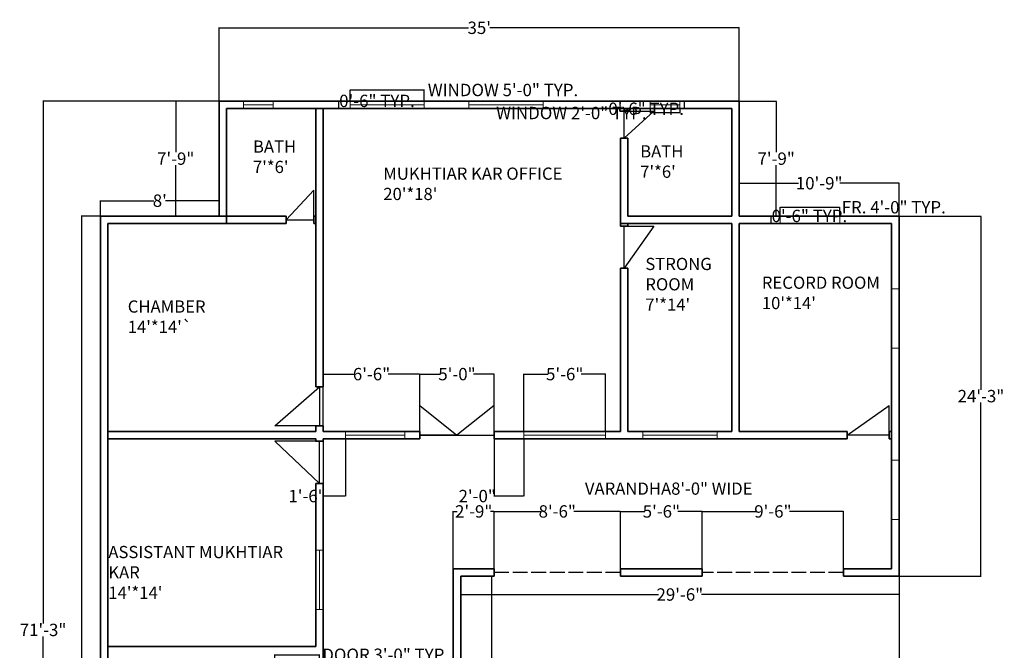
# Model space of a CAD drawing. Units: inches. Extents: x 20 to 815, y -31 to 943.
# Tile 2 of 2: x 20 to 815, y 433 to 943. Entities that reach past the tile are written whole.
import ezdxf

# ---------------------------------------------------------------- set-up
doc = ezdxf.new("R2010")
doc.units = ezdxf.units.IN
doc.header["$MEASUREMENT"] = 0
doc.linetypes.add('ACAD_ISO02W100', pattern=[15, 12, -3])
for name, color, linetype, lineweight in [('A-ANNO-DIMS', 2, 'Continuous', 18), ('A-AREA-IDEN', 7, 'Continuous', 18), ('A-DOOR', 3, 'Continuous', 25), ('A-FLOR-GRIL', 8, 'ACAD_ISO02W100', 25), ('A-GLAZ', 4, 'Continuous', 18), ('A-WALL', 7, 'Continuous', 35)]:
    doc.layers.add(name, color=color, linetype=linetype, lineweight=lineweight)
doc.styles.get("Standard").update_dxf_attribs({"font": 'arial.ttf'})
doc.dimstyles.get("Standard").update_dxf_attribs({"dimtxt": 10, "dimasz": 0.18, "dimexe": 0.18, "dimexo": 0.0625, "dimgap": 0.09, "dimtad": 0, "dimtih": 1, "dimtoh": 1, "dimdec": 0, "dimzin": 0, "dimdsep": 46, "dimlunit": 3, "dimtxsty": 'Standard', "dimcen": 0.09, "dimadec": 0, "dimazin": 0, "dimtfac": 1, "dimtdec": 0, "dimtofl": 0, "dimtmove": 0, "dimatfit": 3, "dimfxl": 1, "dimtolj": 1, "dimtzin": 0, "dimarcsym": 0})

# ---------------------------------------------------------------- blocks, each defined once
blk = doc.blocks.new('*D1')
at = {"layer": 'A-ANNO-DIMS', "color": 0, "lineweight": -2, "transparency": 16777216}
for p, q in [((181.05, 877.05), (181.05, 936.45)), ((181.23, 936.27), (382.48, 936.27)), ((600.87, 936.27), (399.62, 936.27)), ((601.05, 877.05), (601.05, 936.45))]:
    blk.add_line(p, q, dxfattribs=at)
at = {"layer": 'A-ANNO-DIMS', "color": 0, "transparency": 16777216}
for points in [[(181.23, 936.3), (181.23, 936.24), (181.05, 936.27)], [(600.87, 936.3), (600.87, 936.24), (601.05, 936.27)]]:
    blk.add_solid(points, dxfattribs=at)
at = {"layer": 'Defpoints', "color": 0, "transparency": 16777216}
for p in [(601.05, 936.27), (181.05, 876.99), (601.05, 876.99)]:
    blk.add_point(p, dxfattribs=at)
at = {"layer": 'A-ANNO-DIMS', "color": 0, "transparency": 16777216, "insert": (391.05, 936.27), "char_height": 10, "attachment_point": 5}
blk.add_mtext("\\A1;35'", dxfattribs=at)
blk = doc.blocks.new('*D2')
at = {"layer": 'A-ANNO-DIMS', "color": 0, "lineweight": -2, "transparency": 16777216}
for p, q in [((601.11, 876.99), (631.03, 876.99)), ((630.85, 876.81), (630.85, 835.69)), ((630.85, 784.17), (630.85, 825.3)), ((601.11, 783.99), (631.03, 783.99))]:
    blk.add_line(p, q, dxfattribs=at)
at = {"layer": 'A-ANNO-DIMS', "color": 0, "transparency": 16777216}
for points in [[(630.82, 876.81), (630.88, 876.81), (630.85, 876.99)], [(630.82, 784.17), (630.88, 784.17), (630.85, 783.99)]]:
    blk.add_solid(points, dxfattribs=at)
at = {"layer": 'Defpoints', "color": 0, "transparency": 16777216}
for p in [(601.05, 876.99), (601.05, 783.99), (630.85, 783.99)]:
    blk.add_point(p, dxfattribs=at)
at = {"layer": 'A-ANNO-DIMS', "color": 0, "transparency": 16777216, "insert": (630.85, 830.49), "char_height": 10, "attachment_point": 5}
blk.add_mtext('\\A1;7\'-9"', dxfattribs=at)
blk = doc.blocks.new('*D3')
at = {"layer": 'A-ANNO-DIMS', "color": 0, "lineweight": -2, "transparency": 16777216}
for p, q in [((601.05, 784.05), (601.05, 810.82)), ((601.23, 810.64), (648.76, 810.64)), ((729.87, 810.64), (682.35, 810.64)), ((730.05, 784.05), (730.05, 810.82))]:
    blk.add_line(p, q, dxfattribs=at)
at = {"layer": 'A-ANNO-DIMS', "color": 0, "transparency": 16777216}
for points in [[(601.23, 810.67), (601.23, 810.61), (601.05, 810.64)], [(729.87, 810.67), (729.87, 810.61), (730.05, 810.64)]]:
    blk.add_solid(points, dxfattribs=at)
at = {"layer": 'Defpoints', "color": 0, "transparency": 16777216}
for p in [(730.05, 810.64), (601.05, 783.99), (730.05, 783.99)]:
    blk.add_point(p, dxfattribs=at)
at = {"layer": 'A-ANNO-DIMS', "color": 0, "transparency": 16777216, "insert": (665.55, 810.64), "char_height": 10, "attachment_point": 5}
blk.add_mtext('\\A1;10\'-9"', dxfattribs=at)
blk = doc.blocks.new('*D4')
at = {"layer": 'A-ANNO-DIMS', "color": 0, "lineweight": -2, "transparency": 16777216}
for p, q in [((730.11, 783.99), (796.4, 783.99)), ((796.22, 783.81), (796.22, 643.69)), ((796.22, 493.17), (796.22, 633.29)), ((730.11, 492.99), (796.4, 492.99))]:
    blk.add_line(p, q, dxfattribs=at)
at = {"layer": 'A-ANNO-DIMS', "color": 0, "transparency": 16777216}
for points in [[(796.19, 783.81), (796.25, 783.81), (796.22, 783.99)], [(796.19, 493.17), (796.25, 493.17), (796.22, 492.99)]]:
    blk.add_solid(points, dxfattribs=at)
at = {"layer": 'Defpoints', "color": 0, "transparency": 16777216}
for p in [(730.05, 783.99), (796.22, 783.99), (730.05, 492.99)]:
    blk.add_point(p, dxfattribs=at)
at = {"layer": 'A-ANNO-DIMS', "color": 0, "transparency": 16777216, "insert": (796.22, 638.49), "char_height": 10, "attachment_point": 5}
blk.add_mtext('\\A1;24\'-3"', dxfattribs=at)
blk = doc.blocks.new('*D5')
at = {"layer": 'A-ANNO-DIMS', "color": 0, "lineweight": -2, "transparency": 16777216}
for p, q in [((376.05, 492.93), (376.05, 477.94)), ((730.05, 492.93), (730.05, 477.94)), ((376.23, 478.12), (535.7, 478.12)), ((729.87, 478.12), (570.4, 478.12))]:
    blk.add_line(p, q, dxfattribs=at)
at = {"layer": 'A-ANNO-DIMS', "color": 0, "transparency": 16777216}
for points in [[(376.23, 478.15), (376.23, 478.09), (376.05, 478.12)], [(729.87, 478.15), (729.87, 478.09), (730.05, 478.12)]]:
    blk.add_solid(points, dxfattribs=at)
at = {"layer": 'Defpoints', "color": 0, "transparency": 16777216}
for p in [(376.05, 492.99), (730.05, 492.99), (376.05, 478.12)]:
    blk.add_point(p, dxfattribs=at)
at = {"layer": 'A-ANNO-DIMS', "color": 0, "transparency": 16777216, "insert": (553.05, 478.12), "char_height": 10, "attachment_point": 5}
blk.add_mtext('\\A1;29\'-6"', dxfattribs=at)
blk = doc.blocks.new('*D6')
at = {"layer": 'A-ANNO-DIMS', "color": 0, "lineweight": -2, "transparency": 16777216}
for p, q in [((84.99, 783.99), (69.56, 783.99)), ((69.74, 783.81), (69.74, 408.19)), ((69.74, 22.17), (69.74, 397.79)), ((84.99, 21.99), (69.56, 21.99))]:
    blk.add_line(p, q, dxfattribs=at)
at = {"layer": 'A-ANNO-DIMS', "color": 0, "transparency": 16777216}
for points in [[(69.71, 783.81), (69.77, 783.81), (69.74, 783.99)], [(69.71, 22.17), (69.77, 22.17), (69.74, 21.99)]]:
    blk.add_solid(points, dxfattribs=at)
at = {"layer": 'Defpoints', "color": 0, "transparency": 16777216}
for p in [(69.74, 783.99), (85.05, 783.99), (85.05, 21.99)]:
    blk.add_point(p, dxfattribs=at)
at = {"layer": 'A-ANNO-DIMS', "color": 0, "transparency": 16777216, "insert": (69.74, 402.99), "char_height": 10, "attachment_point": 5}
blk.add_mtext('\\A1;63\'-6"', dxfattribs=at)
blk = doc.blocks.new('*D7')
at = {"layer": 'A-ANNO-DIMS', "color": 0, "lineweight": -2, "transparency": 16777216}
for p, q in [((85.05, 784.05), (85.05, 796.69)), ((85.23, 796.51), (128.35, 796.51)), ((180.87, 796.51), (137.75, 796.51)), ((181.05, 784.05), (181.05, 796.69))]:
    blk.add_line(p, q, dxfattribs=at)
at = {"layer": 'A-ANNO-DIMS', "color": 0, "transparency": 16777216}
for points in [[(85.23, 796.54), (85.23, 796.48), (85.05, 796.51)], [(180.87, 796.54), (180.87, 796.48), (181.05, 796.51)]]:
    blk.add_solid(points, dxfattribs=at)
at = {"layer": 'Defpoints', "color": 0, "transparency": 16777216}
for p in [(181.05, 796.51), (85.05, 783.99), (181.05, 783.99)]:
    blk.add_point(p, dxfattribs=at)
at = {"layer": 'A-ANNO-DIMS', "color": 0, "transparency": 16777216, "insert": (133.05, 796.51), "char_height": 10, "attachment_point": 5}
blk.add_mtext("\\A1;8'", dxfattribs=at)
blk = doc.blocks.new('*D8')
at = {"layer": 'A-ANNO-DIMS', "color": 0, "lineweight": -2, "transparency": 16777216}
for p, q in [((180.99, 876.99), (145.7, 876.99)), ((145.88, 876.81), (145.88, 835.69)), ((145.88, 784.17), (145.88, 825.3)), ((180.99, 783.99), (145.7, 783.99))]:
    blk.add_line(p, q, dxfattribs=at)
at = {"layer": 'A-ANNO-DIMS', "color": 0, "transparency": 16777216}
for points in [[(145.85, 876.81), (145.91, 876.81), (145.88, 876.99)], [(145.85, 784.17), (145.91, 784.17), (145.88, 783.99)]]:
    blk.add_solid(points, dxfattribs=at)
at = {"layer": 'Defpoints', "color": 0, "transparency": 16777216}
for p in [(145.88, 876.99), (181.05, 876.99), (181.05, 783.99)]:
    blk.add_point(p, dxfattribs=at)
at = {"layer": 'A-ANNO-DIMS', "color": 0, "transparency": 16777216, "insert": (145.88, 830.49), "char_height": 10, "attachment_point": 5}
blk.add_mtext('\\A1;7\'-9"', dxfattribs=at)
blk = doc.blocks.new('*D9')
at = {"layer": 'A-ANNO-DIMS', "color": 0, "lineweight": -2, "transparency": 16777216}
for p, q in [((376.11, 492.99), (401.14, 492.99)), ((400.96, 492.81), (400.96, 262.69)), ((400.96, 22.17), (400.96, 252.29)), ((376.11, 21.99), (401.14, 21.99))]:
    blk.add_line(p, q, dxfattribs=at)
at = {"layer": 'A-ANNO-DIMS', "color": 0, "transparency": 16777216}
for points in [[(400.93, 492.81), (400.99, 492.81), (400.96, 492.99)], [(400.93, 22.17), (400.99, 22.17), (400.96, 21.99)]]:
    blk.add_solid(points, dxfattribs=at)
at = {"layer": 'Defpoints', "color": 0, "transparency": 16777216}
for p in [(376.05, 492.99), (376.05, 21.99), (400.96, 21.99)]:
    blk.add_point(p, dxfattribs=at)
at = {"layer": 'A-ANNO-DIMS', "color": 0, "transparency": 16777216, "insert": (400.96, 257.49), "char_height": 10, "attachment_point": 5}
blk.add_mtext('\\A1;39\'-3"', dxfattribs=at)
blk = doc.blocks.new('WIN-48')
for p, q in [((-3, 48), (3, 48)), ((0, 0), (0, 48)), ((-3, 0), (3, 0))]:
    blk.add_line(p, q)
blk = doc.blocks.new('WIN-60')
for p, q in [((0, 3), (0, -3)), ((0, 0), (60, 0)), ((60, 3), (60, -3))]:
    blk.add_line(p, q)
blk = doc.blocks.new('WIN-24')
for p, q in [((0, -3), (0, 3)), ((0, 0), (24, 0)), ((24, 3), (24, -3))]:
    blk.add_line(p, q)
blk = doc.blocks.new('WIN-48-FRAME')
for p, q in [((0, 0), (0, 6)), ((0, 6), (48, 6)), ((48, 6), (48, 0))]:
    blk.add_line(p, q)
blk = doc.blocks.new('*D18')
at = {"layer": 'A-ANNO-DIMS', "color": 0, "lineweight": -2, "transparency": 16777216}
for p, q in [((286.68, 877.05), (286.68, 886.17)), ((286.86, 885.99), (346.5, 885.99)), ((346.68, 877.05), (346.68, 886.17)), ((346.68, 885.99), (346.86, 885.99))]:
    blk.add_line(p, q, dxfattribs=at)
at = {"layer": 'A-ANNO-DIMS', "color": 0, "transparency": 16777216}
for points in [[(286.86, 886.02), (286.86, 885.96), (286.68, 885.99)], [(346.5, 886.02), (346.5, 885.96), (346.68, 885.99)]]:
    blk.add_solid(points, dxfattribs=at)
at = {"layer": 'Defpoints', "color": 0, "transparency": 16777216}
for p in [(346.68, 885.99), (286.68, 876.99), (346.68, 876.99)]:
    blk.add_point(p, dxfattribs=at)
at = {"layer": 'A-ANNO-DIMS', "color": 0, "transparency": 16777216, "insert": (410.22, 885.99), "char_height": 10, "attachment_point": 5}
blk.add_mtext('\\A1;WINDOW 5\'-0" TYP.', dxfattribs=at)
blk = doc.blocks.new('*D19')
at = {"layer": 'A-ANNO-DIMS', "color": 0, "lineweight": -2, "transparency": 16777216}
for p, q in [((286.62, 876.99), (277.5, 876.99)), ((277.68, 876.99), (277.68, 877.17)), ((277.68, 877.17), (277.86, 877.17)), ((277.68, 871.17), (277.68, 876.81)), ((286.62, 870.99), (277.5, 870.99))]:
    blk.add_line(p, q, dxfattribs=at)
at = {"layer": 'A-ANNO-DIMS', "color": 0, "transparency": 16777216}
for points in [[(277.65, 876.81), (277.71, 876.81), (277.68, 876.99)], [(277.65, 871.17), (277.71, 871.17), (277.68, 870.99)]]:
    blk.add_solid(points, dxfattribs=at)
at = {"layer": 'Defpoints', "color": 0, "transparency": 16777216}
for p in [(277.68, 876.99), (286.68, 876.99), (286.68, 870.99)]:
    blk.add_point(p, dxfattribs=at)
at = {"layer": 'A-ANNO-DIMS', "color": 0, "transparency": 16777216, "insert": (308.43, 877.17), "char_height": 10, "attachment_point": 5}
blk.add_mtext('\\A1;0\'-6" TYP.', dxfattribs=at)
blk = doc.blocks.new('*D20')
at = {"layer": 'A-ANNO-DIMS', "color": 0, "lineweight": -2, "transparency": 16777216}
for p, q in [((528.98, 867.39), (528.8, 867.39)), ((528.98, 870.93), (528.98, 867.21)), ((552.8, 867.39), (529.16, 867.39)), ((552.98, 870.93), (552.98, 867.21))]:
    blk.add_line(p, q, dxfattribs=at)
at = {"layer": 'A-ANNO-DIMS', "color": 0, "transparency": 16777216}
for points in [[(529.16, 867.42), (529.16, 867.36), (528.98, 867.39)], [(552.8, 867.42), (552.8, 867.36), (552.98, 867.39)]]:
    blk.add_solid(points, dxfattribs=at)
at = {"layer": 'Defpoints', "color": 0, "transparency": 16777216}
for p in [(528.98, 870.99), (528.98, 867.39), (552.98, 870.99)]:
    blk.add_point(p, dxfattribs=at)
at = {"layer": 'A-ANNO-DIMS', "color": 0, "transparency": 16777216, "insert": (465.43, 867.39), "char_height": 10, "attachment_point": 5}
blk.add_mtext('\\A1;WINDOW 2\'-0" TYP.', dxfattribs=at)
blk = doc.blocks.new('*D21')
at = {"layer": 'A-ANNO-DIMS', "color": 0, "lineweight": -2, "transparency": 16777216}
for p, q in [((553.04, 876.99), (556.76, 876.99)), ((556.58, 876.81), (556.58, 871.17)), ((553.04, 870.99), (556.76, 870.99)), ((556.58, 870.81), (556.4, 870.81)), ((556.58, 870.99), (556.58, 870.81))]:
    blk.add_line(p, q, dxfattribs=at)
at = {"layer": 'A-ANNO-DIMS', "color": 0, "transparency": 16777216}
for points in [[(556.55, 876.81), (556.61, 876.81), (556.58, 876.99)], [(556.55, 871.17), (556.61, 871.17), (556.58, 870.99)]]:
    blk.add_solid(points, dxfattribs=at)
at = {"layer": 'Defpoints', "color": 0, "transparency": 16777216}
for p in [(552.98, 876.99), (552.98, 870.99), (556.58, 870.99)]:
    blk.add_point(p, dxfattribs=at)
at = {"layer": 'A-ANNO-DIMS', "color": 0, "transparency": 16777216, "insert": (525.83, 870.81), "char_height": 10, "attachment_point": 5}
blk.add_mtext('\\A1;0\'-6" TYP.', dxfattribs=at)
blk = doc.blocks.new('*D22')
at = {"layer": 'A-ANNO-DIMS', "color": 0, "lineweight": -2, "transparency": 16777216}
for p, q in [((634.12, 784.05), (634.12, 791.37)), ((634.3, 791.19), (681.94, 791.19)), ((682.12, 784.05), (682.12, 791.37)), ((682.12, 791.19), (682.3, 791.19))]:
    blk.add_line(p, q, dxfattribs=at)
at = {"layer": 'A-ANNO-DIMS', "color": 0, "transparency": 16777216}
for points in [[(634.3, 791.22), (634.3, 791.16), (634.12, 791.19)], [(681.94, 791.22), (681.94, 791.16), (682.12, 791.19)]]:
    blk.add_solid(points, dxfattribs=at)
at = {"layer": 'Defpoints', "color": 0, "transparency": 16777216}
for p in [(682.12, 791.19), (634.12, 783.99), (682.12, 783.99)]:
    blk.add_point(p, dxfattribs=at)
at = {"layer": 'A-ANNO-DIMS', "color": 0, "transparency": 16777216, "insert": (725.77, 791.19), "char_height": 10, "attachment_point": 5}
blk.add_mtext('\\A1;FR. 4\'-0" TYP.', dxfattribs=at)
blk = doc.blocks.new('*D23')
at = {"layer": 'A-ANNO-DIMS', "color": 0, "lineweight": -2, "transparency": 16777216}
for p, q in [((634.05, 783.99), (626.74, 783.99)), ((626.92, 783.99), (626.92, 784.17)), ((626.92, 784.17), (627.1, 784.17)), ((626.92, 778.17), (626.92, 783.81)), ((634.05, 777.99), (626.74, 777.99))]:
    blk.add_line(p, q, dxfattribs=at)
at = {"layer": 'A-ANNO-DIMS', "color": 0, "transparency": 16777216}
for points in [[(626.89, 783.81), (626.95, 783.81), (626.92, 783.99)], [(626.89, 778.17), (626.95, 778.17), (626.92, 777.99)]]:
    blk.add_solid(points, dxfattribs=at)
at = {"layer": 'Defpoints', "color": 0, "transparency": 16777216}
for p in [(626.92, 783.99), (634.12, 783.99), (634.12, 777.99)]:
    blk.add_point(p, dxfattribs=at)
at = {"layer": 'A-ANNO-DIMS', "color": 0, "transparency": 16777216, "insert": (657.66, 784.17), "char_height": 10, "attachment_point": 5}
blk.add_mtext('\\A1;0\'-6" TYP.', dxfattribs=at)
blk = doc.blocks.new('*D24')
at = {"layer": 'A-ANNO-DIMS', "color": 0, "lineweight": -2, "transparency": 16777216}
for p, q in [((226.05, 424.05), (226.05, 429.57)), ((262.05, 424.05), (262.05, 429.57)), ((226.23, 429.39), (261.87, 429.39)), ((262.05, 429.39), (262.23, 429.39))]:
    blk.add_line(p, q, dxfattribs=at)
at = {"layer": 'A-ANNO-DIMS', "color": 0, "transparency": 16777216}
for points in [[(226.23, 429.42), (226.23, 429.36), (226.05, 429.39)], [(261.87, 429.42), (261.87, 429.36), (262.05, 429.39)]]:
    blk.add_solid(points, dxfattribs=at)
at = {"layer": 'Defpoints', "color": 0, "transparency": 16777216}
for p in [(226.05, 423.99), (262.05, 429.39), (262.05, 423.99)]:
    blk.add_point(p, dxfattribs=at)
at = {"layer": 'A-ANNO-DIMS', "color": 0, "transparency": 16777216, "insert": (315.45, 429.39), "char_height": 10, "attachment_point": 5}
blk.add_mtext('\\A1;DOOR 3\'-0" TYP.', dxfattribs=at)
blk = doc.blocks.new('*D28')
at = {"layer": 'A-ANNO-DIMS', "color": 0, "lineweight": -2, "transparency": 16777216}
for p, q in [((730.05, 492.93), (730.05, -24.49)), ((85.05, 21.93), (85.05, -24.49)), ((85.23, -24.31), (390.29, -24.31)), ((729.87, -24.31), (424.82, -24.31))]:
    blk.add_line(p, q, dxfattribs=at)
at = {"layer": 'A-ANNO-DIMS', "color": 0, "transparency": 16777216}
for points in [[(85.23, -24.28), (85.23, -24.34), (85.05, -24.31)], [(729.87, -24.28), (729.87, -24.34), (730.05, -24.31)]]:
    blk.add_solid(points, dxfattribs=at)
at = {"layer": 'Defpoints', "color": 0, "transparency": 16777216}
for p in [(730.05, 492.99), (85.05, 21.99), (730.05, -24.31)]:
    blk.add_point(p, dxfattribs=at)
at = {"layer": 'A-ANNO-DIMS', "color": 0, "transparency": 16777216, "insert": (407.55, -24.31), "char_height": 10, "attachment_point": 5}
blk.add_mtext('\\A1;53\'-9"', dxfattribs=at)
blk = doc.blocks.new('*D29')
at = {"layer": 'A-ANNO-DIMS', "color": 0, "lineweight": -2, "transparency": 16777216}
for p, q in [((180.99, 876.99), (38.57, 876.99)), ((38.75, 876.81), (38.75, 454.69)), ((38.75, 22.17), (38.75, 444.29)), ((84.99, 21.99), (38.57, 21.99))]:
    blk.add_line(p, q, dxfattribs=at)
at = {"layer": 'A-ANNO-DIMS', "color": 0, "transparency": 16777216}
for points in [[(38.72, 876.81), (38.78, 876.81), (38.75, 876.99)], [(38.72, 22.17), (38.78, 22.17), (38.75, 21.99)]]:
    blk.add_solid(points, dxfattribs=at)
at = {"layer": 'Defpoints', "color": 0, "transparency": 16777216}
for p in [(38.75, 876.99), (181.05, 876.99), (85.05, 21.99)]:
    blk.add_point(p, dxfattribs=at)
at = {"layer": 'A-ANNO-DIMS', "color": 0, "transparency": 16777216, "insert": (38.75, 449.49), "char_height": 10, "attachment_point": 5}
blk.add_mtext('\\A1;71\'-3"', dxfattribs=at)
blk = doc.blocks.new('*D34')
at = {"layer": 'A-ANNO-DIMS', "color": 0, "lineweight": -2, "transparency": 16777216}
for p, q in [((370.05, 499.05), (370.05, 545.47)), ((370.23, 545.29), (373.08, 545.29)), ((402.87, 545.29), (400.02, 545.29)), ((403.05, 499.05), (403.05, 545.47))]:
    blk.add_line(p, q, dxfattribs=at)
at = {"layer": 'A-ANNO-DIMS', "color": 0, "transparency": 16777216}
for points in [[(370.23, 545.32), (370.23, 545.26), (370.05, 545.29)], [(402.87, 545.32), (402.87, 545.26), (403.05, 545.29)]]:
    blk.add_solid(points, dxfattribs=at)
at = {"layer": 'Defpoints', "color": 0, "transparency": 16777216}
for p in [(403.05, 545.29), (370.05, 498.99), (403.05, 498.99)]:
    blk.add_point(p, dxfattribs=at)
at = {"layer": 'A-ANNO-DIMS', "color": 0, "transparency": 16777216, "insert": (386.55, 545.29), "char_height": 10, "attachment_point": 5}
blk.add_mtext('\\A1;2\'-9"', dxfattribs=at)
blk = doc.blocks.new('*D35')
at = {"layer": 'A-ANNO-DIMS', "color": 0, "lineweight": -2, "transparency": 16777216}
for p, q in [((403.05, 499.05), (403.05, 545.47)), ((403.23, 545.29), (440.66, 545.29)), ((504.87, 545.29), (467.44, 545.29)), ((505.05, 499.05), (505.05, 545.47))]:
    blk.add_line(p, q, dxfattribs=at)
at = {"layer": 'A-ANNO-DIMS', "color": 0, "transparency": 16777216}
for points in [[(403.23, 545.32), (403.23, 545.26), (403.05, 545.29)], [(504.87, 545.32), (504.87, 545.26), (505.05, 545.29)]]:
    blk.add_solid(points, dxfattribs=at)
at = {"layer": 'Defpoints', "color": 0, "transparency": 16777216}
for p in [(505.05, 545.29), (403.05, 498.99), (505.05, 498.99)]:
    blk.add_point(p, dxfattribs=at)
at = {"layer": 'A-ANNO-DIMS', "color": 0, "transparency": 16777216, "insert": (454.05, 545.29), "char_height": 10, "attachment_point": 5}
blk.add_mtext('\\A1;8\'-6"', dxfattribs=at)
blk = doc.blocks.new('*D36')
at = {"layer": 'A-ANNO-DIMS', "color": 0, "lineweight": -2, "transparency": 16777216}
for p, q in [((505.05, 499.05), (505.05, 545.47)), ((505.23, 545.29), (524.74, 545.29)), ((571.02, 545.29), (551.51, 545.29)), ((571.2, 499.05), (571.2, 545.47))]:
    blk.add_line(p, q, dxfattribs=at)
at = {"layer": 'A-ANNO-DIMS', "color": 0, "transparency": 16777216}
for points in [[(505.23, 545.32), (505.23, 545.26), (505.05, 545.29)], [(571.02, 545.32), (571.02, 545.26), (571.2, 545.29)]]:
    blk.add_solid(points, dxfattribs=at)
at = {"layer": 'Defpoints', "color": 0, "transparency": 16777216}
for p in [(571.2, 545.29), (505.05, 498.99), (571.2, 498.99)]:
    blk.add_point(p, dxfattribs=at)
at = {"layer": 'A-ANNO-DIMS', "color": 0, "transparency": 16777216, "insert": (538.12, 545.29), "char_height": 10, "attachment_point": 5}
blk.add_mtext('\\A1;5\'-6"', dxfattribs=at)
blk = doc.blocks.new('*D37')
at = {"layer": 'A-ANNO-DIMS', "color": 0, "lineweight": -2, "transparency": 16777216}
for p, q in [((571.2, 499.05), (571.2, 545.47)), ((571.38, 545.29), (614.81, 545.29)), ((685.01, 545.29), (641.58, 545.29)), ((685.19, 499.05), (685.19, 545.47))]:
    blk.add_line(p, q, dxfattribs=at)
at = {"layer": 'A-ANNO-DIMS', "color": 0, "transparency": 16777216}
for points in [[(571.38, 545.32), (571.38, 545.26), (571.2, 545.29)], [(685.01, 545.32), (685.01, 545.26), (685.19, 545.29)]]:
    blk.add_solid(points, dxfattribs=at)
at = {"layer": 'Defpoints', "color": 0, "transparency": 16777216}
for p in [(685.19, 545.29), (571.2, 498.99), (685.19, 498.99)]:
    blk.add_point(p, dxfattribs=at)
at = {"layer": 'A-ANNO-DIMS', "color": 0, "transparency": 16777216, "insert": (628.19, 545.29), "char_height": 10, "attachment_point": 5}
blk.add_mtext('\\A1;9\'-6"', dxfattribs=at)
blk = doc.blocks.new('*D38')
at = {"layer": 'A-ANNO-DIMS', "color": 0, "lineweight": -2, "transparency": 16777216}
for p, q in [((265.05, 610.05), (265.05, 656.47)), ((265.23, 656.29), (290.64, 656.29)), ((342.87, 656.29), (317.46, 656.29)), ((343.05, 610.05), (343.05, 656.47))]:
    blk.add_line(p, q, dxfattribs=at)
at = {"layer": 'A-ANNO-DIMS', "color": 0, "transparency": 16777216}
for points in [[(265.23, 656.32), (265.23, 656.26), (265.05, 656.29)], [(342.87, 656.32), (342.87, 656.26), (343.05, 656.29)]]:
    blk.add_solid(points, dxfattribs=at)
at = {"layer": 'Defpoints', "color": 0, "transparency": 16777216}
for p in [(343.05, 656.29), (265.05, 609.99), (343.05, 609.99)]:
    blk.add_point(p, dxfattribs=at)
at = {"layer": 'A-ANNO-DIMS', "color": 0, "transparency": 16777216, "insert": (304.05, 656.29), "char_height": 10, "attachment_point": 5}
blk.add_mtext('\\A1;6\'-6"', dxfattribs=at)
blk = doc.blocks.new('*D39')
at = {"layer": 'A-ANNO-DIMS', "color": 0, "lineweight": -2, "transparency": 16777216}
for p, q in [((343.05, 610.05), (343.05, 656.47)), ((343.23, 656.29), (359.67, 656.29)), ((402.87, 656.29), (386.43, 656.29)), ((403.05, 610.05), (403.05, 656.47))]:
    blk.add_line(p, q, dxfattribs=at)
at = {"layer": 'A-ANNO-DIMS', "color": 0, "transparency": 16777216}
for points in [[(343.23, 656.32), (343.23, 656.26), (343.05, 656.29)], [(402.87, 656.32), (402.87, 656.26), (403.05, 656.29)]]:
    blk.add_solid(points, dxfattribs=at)
at = {"layer": 'Defpoints', "color": 0, "transparency": 16777216}
for p in [(403.05, 656.29), (343.05, 609.99), (403.05, 609.99)]:
    blk.add_point(p, dxfattribs=at)
at = {"layer": 'A-ANNO-DIMS', "color": 0, "transparency": 16777216, "insert": (373.05, 656.29), "char_height": 10, "attachment_point": 5}
blk.add_mtext('\\A1;5\'-0"', dxfattribs=at)
blk = doc.blocks.new('*D40')
at = {"layer": 'A-ANNO-DIMS', "color": 0, "lineweight": -2, "transparency": 16777216}
for p, q in [((403.05, 603.93), (403.05, 557.51)), ((427.05, 603.93), (427.05, 557.51)), ((403.05, 557.69), (402.87, 557.69)), ((426.87, 557.69), (403.23, 557.69))]:
    blk.add_line(p, q, dxfattribs=at)
at = {"layer": 'A-ANNO-DIMS', "color": 0, "transparency": 16777216}
for points in [[(403.23, 557.72), (403.23, 557.66), (403.05, 557.69)], [(426.87, 557.72), (426.87, 557.66), (427.05, 557.69)]]:
    blk.add_solid(points, dxfattribs=at)
at = {"layer": 'Defpoints', "color": 0, "transparency": 16777216}
for p in [(403.05, 603.99), (427.05, 603.99), (403.05, 557.69)]:
    blk.add_point(p, dxfattribs=at)
at = {"layer": 'A-ANNO-DIMS', "color": 0, "transparency": 16777216, "insert": (389.4, 557.69), "char_height": 10, "attachment_point": 5}
blk.add_mtext('\\A1;2\'-0"', dxfattribs=at)
blk = doc.blocks.new('*D41')
at = {"layer": 'A-ANNO-DIMS', "color": 0, "lineweight": -2, "transparency": 16777216}
for p, q in [((427.05, 610.05), (427.05, 656.47)), ((427.23, 656.29), (446.67, 656.29)), ((492.87, 656.29), (473.43, 656.29)), ((493.05, 610.05), (493.05, 656.47))]:
    blk.add_line(p, q, dxfattribs=at)
at = {"layer": 'A-ANNO-DIMS', "color": 0, "transparency": 16777216}
for points in [[(427.23, 656.32), (427.23, 656.26), (427.05, 656.29)], [(492.87, 656.32), (492.87, 656.26), (493.05, 656.29)]]:
    blk.add_solid(points, dxfattribs=at)
at = {"layer": 'Defpoints', "color": 0, "transparency": 16777216}
for p in [(493.05, 656.29), (427.05, 609.99), (493.05, 609.99)]:
    blk.add_point(p, dxfattribs=at)
at = {"layer": 'A-ANNO-DIMS', "color": 0, "transparency": 16777216, "insert": (460.05, 656.29), "char_height": 10, "attachment_point": 5}
blk.add_mtext('\\A1;5\'-6"', dxfattribs=at)
blk = doc.blocks.new('*D42')
at = {"layer": 'A-ANNO-DIMS', "color": 0, "lineweight": -2, "transparency": 16777216}
for p, q in [((265.05, 603.93), (265.05, 557.51)), ((283.05, 603.93), (283.05, 557.51)), ((265.05, 557.69), (264.87, 557.69)), ((282.87, 557.69), (265.23, 557.69))]:
    blk.add_line(p, q, dxfattribs=at)
at = {"layer": 'A-ANNO-DIMS', "color": 0, "transparency": 16777216}
for points in [[(265.23, 557.72), (265.23, 557.66), (265.05, 557.69)], [(282.87, 557.72), (282.87, 557.66), (283.05, 557.69)]]:
    blk.add_solid(points, dxfattribs=at)
at = {"layer": 'Defpoints', "color": 0, "transparency": 16777216}
for p in [(265.05, 603.99), (283.05, 603.99), (265.05, 557.69)]:
    blk.add_point(p, dxfattribs=at)
at = {"layer": 'A-ANNO-DIMS', "color": 0, "transparency": 16777216, "insert": (251.96, 557.69), "char_height": 10, "attachment_point": 5}
blk.add_mtext('\\A1;1\'-6"', dxfattribs=at)

msp = doc.modelspace()

# ---------------------------------------------------------------- linework, layer by layer
at = {"layer": 'A-DOOR'}
for p, q in [((508.05, 846.99), (508.05, 868.99)), ((508.05, 868.99), (532.05, 868.99)), ((532.05, 868.99), (508.05, 846.99)), ((257.49, 804.99), (235.05, 780.99)), ((257.49, 780.99), (257.49, 804.99)), ((235.05, 780.99), (257.49, 780.99)), ((226.05, 614.4), (262.05, 645.99)), ((262.05, 645.99), (262.05, 614.4)), ((343.06, 606.99), (343.06, 630.99)), ((343.06, 630.99), (373.05, 606.99)), ((403.05, 630.99), (373.05, 606.99)), ((403.05, 606.99), (403.05, 630.99)), ((688.05, 606.99), (722.05, 630.99)), ((722.05, 606.99), (722.05, 630.99)), ((262.05, 614.4), (226.05, 614.4)), ((343.05, 606.99), (403.05, 606.99)), ((373.05, 606.99), (343.06, 606.99)), ((722.05, 606.99), (688.05, 606.99)), ((262.05, 601.99), (226.05, 601.99)), ((226.05, 601.99), (262.05, 567.99)), ((262.05, 567.99), (262.05, 601.99))]:
    msp.add_line(p, q, dxfattribs=at)
msp.add_lwpolyline([(508.05, 741.99), (508.05, 775.99), (532.05, 775.99)], close=True, dxfattribs=at)
at = {"layer": 'A-FLOR-GRIL'}
for p, q in [((505.05, 495.99), (403.05, 495.99)), ((685.19, 495.99), (571.2, 495.99))]:
    msp.add_line(p, q, dxfattribs=at)
at = {"layer": 'A-GLAZ'}
for p, q in [((200.66, 876.99), (224.66, 876.99)), ((427.05, 603.99), (427.05, 609.99)), ((427.05, 606.99), (493.05, 606.99)), ((493.05, 603.99), (493.05, 609.99)), ((331.05, 603.99), (283.05, 603.99)), ((724.05, 586.74), (730.05, 586.74)), ((724.05, 538.74), (730.05, 538.74)), ((265.05, 465.99), (265.05, 513.99))]:
    msp.add_line(p, q, dxfattribs=at)
at = {"layer": 'A-WALL'}
for p, q in [((181.05, 783.99), (181.05, 876.99)), ((181.05, 876.99), (601.05, 876.99)), ((601.05, 876.99), (601.05, 783.99)), ((187.05, 777.99), (187.05, 870.99)), ((187.05, 870.99), (595.05, 870.99)), ((259.05, 777.99), (259.05, 870.99)), ((265.05, 645.99), (265.05, 870.99)), ((595.05, 870.99), (595.05, 783.99)), ((595.05, 783.99), (595.05, 870.99)), ((601.05, 783.99), (601.05, 870.99)), ((505.05, 846.99), (511.05, 846.99)), ((505.05, 777.99), (505.05, 846.99)), ((511.05, 783.99), (511.05, 846.99)), ((85.05, 783.99), (181.05, 783.99)), ((85.05, 21.99), (85.05, 783.99)), ((91.05, 783.99), (235.05, 783.99)), ((187.05, 783.99), (235.05, 783.99)), ((235.05, 777.99), (235.05, 783.99)), ((257.49, 777.99), (257.49, 783.99)), ((257.49, 783.99), (259.05, 783.99)), ((265.05, 777.99), (265.05, 783.99)), ((511.05, 783.99), (595.05, 783.99)), ((601.05, 783.99), (730.05, 783.99)), ((730.05, 783.99), (730.05, 492.99)), ((91.05, 777.99), (235.05, 777.99)), ((91.05, 27.99), (91.05, 777.99)), ((187.05, 777.99), (235.05, 777.99)), ((259.05, 777.99), (257.49, 777.99)), ((259.05, 645.99), (259.05, 777.99)), ((505.05, 777.99), (595.05, 777.99)), ((595.05, 609.99), (595.05, 777.99)), ((601.05, 777.99), (724.05, 777.99)), ((601.05, 609.99), (601.05, 777.99)), ((724.05, 777.99), (724.05, 498.99)), ((505.05, 609.99), (505.05, 741.99)), ((505.05, 741.99), (511.05, 741.99)), ((511.05, 609.99), (511.05, 741.99)), ((259.05, 645.99), (265.05, 645.99)), ((265.05, 614.4), (259.05, 614.4)), ((91.05, 609.99), (259.05, 609.99)), ((187.05, 609.99), (259.05, 609.99)), ((265.05, 609.99), (343.05, 609.99)), ((343.05, 603.99), (343.05, 609.99)), ((403.05, 609.99), (505.05, 609.99)), ((403.05, 603.99), (403.05, 609.99)), ((511.05, 609.99), (595.05, 609.99)), ((601.05, 609.99), (688.05, 609.99)), ((688.05, 609.99), (688.05, 603.99)), ((722.05, 603.99), (722.05, 609.99)), ((722.05, 609.99), (724.05, 609.99)), ((91.05, 603.99), (259.05, 603.99)), ((187.05, 603.99), (259.05, 603.99)), ((265.05, 603.99), (343.05, 603.99)), ((403.05, 603.99), (688.05, 603.99)), ((724.05, 603.99), (722.05, 603.99)), ((259.05, 567.99), (265.05, 567.99)), ((259.05, 435.99), (259.05, 567.99)), ((265.05, 423.99), (265.05, 567.99)), ((370.05, 498.99), (370.05, 423.99)), ((403.05, 498.99), (370.05, 498.99)), ((403.05, 492.99), (403.05, 498.99)), ((505.05, 492.99), (505.05, 498.99)), ((571.2, 498.99), (505.05, 498.99)), ((571.2, 492.99), (571.2, 498.99)), ((724.05, 498.99), (685.19, 498.99)), ((685.19, 492.99), (685.19, 498.99)), ((376.05, 492.99), (376.05, 423.99)), ((403.05, 492.99), (376.05, 492.99)), ((571.2, 492.99), (505.05, 492.99)), ((730.05, 492.99), (685.19, 492.99)), ((259.05, 435.99), (259.05, 465.99)), ((91.05, 435.99), (259.05, 435.99))]:
    msp.add_line(p, q, dxfattribs=at)
for points in [[(510.58, 870.99), (510.58, 868.99), (504.62, 868.99), (504.62, 870.99)], [(511, 777.99), (511, 775.99), (505.05, 775.99), (505.05, 777.99)], [(259.05, 614.4), (259.05, 609.99)], [(265.05, 609.99), (265.05, 614.4)], [(259.05, 603.99), (259.05, 603.99), (259.05, 601.99), (265.05, 601.99), (265.05, 603.99)]]:
    msp.add_lwpolyline(points, dxfattribs=at)

# ---------------------------------------------------------------- block references
at = {"layer": 'A-GLAZ'}
for name, p in [('WIN-24', (200.66, 873.99)), ('WIN-60', (286.68, 873.99)), ('WIN-60', (382.68, 873.99)), ('WIN-48-FRAME', (634.12, 777.99)), ('WIN-60', (523.05, 606.99))]:
    msp.add_blockref(name, p, dxfattribs=at)
for name, p, rotation in [('WIN-24', (552.98, 873.99), 180), ('WIN-48-FRAME', (724.05, 725.32), 270.0000000000003), ('WIN-48', (283.05, 606.99), 270.0000000000003), ('WIN-48', (262.05, 513.99), 180)]:
    msp.add_blockref(name, p, dxfattribs=dict(at, rotation=rotation))

# ---------------------------------------------------------------- texts
at = {"layer": 'A-AREA-IDEN', "attachment_point": 1}
for s, insert, char_height in [("BATH\\P7'*6'", (208.28, 845.17), 9.868), ("BATH\\P7'*6'", (521.02, 841.3), 9.868), ("MUKHTIAR KAR OFFICE\\P20'*18'", (313.56, 823.3), 9.8677), ("STRONG\\PROOM\\P7'*14'", (525.17, 750.29), 9.868), ("RECORD ROOM\\P10'*14'", (619.27, 735.12), 9.8677), ("CHAMBER\\P14'*14'`", (107.17, 715.86), 9.868), ('VARANDHA8\'-0" WIDE', (476.38, 568.65), 9.8677), ("ASSISTANT MUKHTIAR\\P                KAR\\P         14'*14'", (91.48, 517.38), 9.8677)]:
    msp.add_mtext(s, dxfattribs=dict(at, insert=insert, char_height=char_height))

# ---------------------------------------------------------------- dimensions: what is measured, and where the dimension line sits
at = {"layer": 'A-ANNO-DIMS'}
for base, p1, p2, override, picture, middle in [((601.05, 936.27), (181.05, 876.99), (601.05, 876.99), {"dimclrd": 0, "dimclre": 0, "dimclrt": 0}, '*D1', (391.05, 936.27)), ((730.05, 810.64), (601.05, 783.99), (730.05, 783.99), {"dimclrd": 0, "dimclre": 0, "dimclrt": 0}, '*D3', (665.55, 810.64)), ((181.05, 796.51), (85.05, 783.99), (181.05, 783.99), {"dimclrd": 0, "dimclre": 0, "dimclrt": 0}, '*D7', (133.05, 796.51)), ((343.05, 656.29), (265.05, 609.99), (343.05, 609.99), {"dimdec": 1, "dimlfac": 1, "dimrnd": 0, "dimzin": 1, "dimdsep": 46, "dimlunit": 4, "dimfrac": 2}, '*D38', (304.05, 656.29)), ((403.05, 656.29), (343.05, 609.99), (403.05, 609.99), {"dimdec": 1, "dimlfac": 1, "dimrnd": 0, "dimzin": 1, "dimdsep": 46, "dimlunit": 4, "dimfrac": 2}, '*D39', (373.05, 656.29)), ((493.05, 656.29), (427.05, 609.99), (493.05, 609.99), {"dimdec": 1, "dimlfac": 1, "dimrnd": 0, "dimzin": 1, "dimdsep": 46, "dimlunit": 4, "dimfrac": 2}, '*D41', (460.05, 656.29)), ((403.05, 545.29), (370.05, 498.99), (403.05, 498.99), {"dimdec": 1, "dimlfac": 1, "dimrnd": 0, "dimzin": 1, "dimdsep": 46, "dimlunit": 4, "dimfrac": 2}, '*D34', (386.55, 545.29)), ((571.1973, 545.2919), (505.0512, 498.9919), (571.1973, 498.9919), {"dimdec": 1, "dimlfac": 1, "dimrnd": 0, "dimzin": 1, "dimdsep": 46, "dimlunit": 4, "dimfrac": 2}, '*D36', (538.1243, 545.2919)), ((685.19, 545.29), (571.2, 498.99), (685.19, 498.99), {"dimdec": 1, "dimlfac": 1, "dimrnd": 0, "dimzin": 1, "dimdsep": 46, "dimlunit": 4, "dimfrac": 2}, '*D37', (628.19, 545.29)), ((730.05, -24.31), (85.05, 21.99), (730.05, 492.99), {"dimdec": 1, "dimlfac": 1, "dimrnd": 0, "dimzin": 1, "dimdsep": 46, "dimlunit": 4, "dimfrac": 2}, '*D28', (407.55, -24.31)), ((376.05, 478.12), (730.05, 492.99), (376.05, 492.99), {"dimclrd": 0, "dimclre": 0, "dimclrt": 0}, '*D5', (553.05, 478.12))]:
    dim = msp.add_linear_dim(base=base, p1=p1, p2=p2, dimstyle='Standard', override=override, dxfattribs=at)
    dim.commit()
    dim.dimension.update_dxf_attribs({"geometry": picture, "text_midpoint": middle})
for base, p1, p2, text, picture, middle in [((346.68, 885.99), (286.68, 876.99), (346.68, 876.99), 'WINDOW <> TYP.', '*D18', (410.22, 885.99)), ((682.12, 791.19), (634.12, 783.99), (682.12, 783.99), 'FR. <> TYP.', '*D22', (725.77, 791.19)), ((262.05, 429.39), (226.05, 423.99), (262.05, 423.99), 'DOOR <> TYP.', '*D24', (315.45, 429.39))]:
    dim = msp.add_linear_dim(base=base, p1=p1, p2=p2, text=text, dimstyle='Standard', override={"dimdec": 1, "dimlfac": 1, "dimrnd": 0, "dimzin": 1, "dimdsep": 46, "dimlunit": 4, "dimfrac": 2}, dxfattribs=at)
    dim.commit()
    dim.dimension.update_dxf_attribs({"geometry": picture, "text_midpoint": middle})
for base, p1, p2, angle, text, picture, middle in [((277.68, 876.99), (286.68, 870.99), (286.68, 876.99), 90, '<> TYP.', '*D19', (308.43, 877.17)), ((528.98, 867.39), (552.98, 870.99), (528.98, 870.99), 180, 'WINDOW <> TYP.', '*D20', (465.43, 867.39)), ((556.58, 870.99), (552.98, 876.99), (552.98, 870.99), 270, '<> TYP.', '*D21', (525.83, 870.81)), ((626.92, 783.99), (634.12, 777.99), (634.12, 783.99), 90, '<> TYP.', '*D23', (657.66, 784.17))]:
    dim = msp.add_linear_dim(base=base, p1=p1, p2=p2, angle=angle, text=text, dimstyle='Standard', override={"dimdec": 1, "dimlfac": 1, "dimrnd": 0, "dimzin": 1, "dimdsep": 46, "dimlunit": 4, "dimfrac": 2}, dxfattribs=at)
    dim.commit()
    dim.dimension.update_dxf_attribs({"geometry": picture, "text_midpoint": middle})
for base, p1, p2, angle, override, picture, middle in [((38.75, 876.99), (85.05, 21.99), (181.05, 876.99), 90, {"dimdec": 1, "dimlfac": 1, "dimrnd": 0, "dimzin": 1, "dimdsep": 46, "dimlunit": 4, "dimfrac": 2}, '*D29', (38.75, 449.49)), ((145.88, 876.99), (181.05, 783.99), (181.05, 876.99), 90, {"dimclrd": 0, "dimclre": 0, "dimclrt": 0}, '*D8', (145.88, 830.49)), ((630.85, 783.99), (601.05, 876.99), (601.05, 783.99), 90, {"dimclrd": 0, "dimclre": 0, "dimclrt": 0}, '*D2', (630.85, 830.49)), ((69.74, 783.99), (85.05, 21.99), (85.05, 783.99), 90, {"dimclrd": 0, "dimclre": 0, "dimclrt": 0}, '*D6', (69.74, 402.99)), ((796.22, 783.99), (730.05, 492.99), (730.05, 783.99), 90, {"dimclrd": 0, "dimclre": 0, "dimclrt": 0}, '*D4', (796.22, 638.49)), ((265.05, 557.69), (283.05, 603.99), (265.05, 603.99), 180, {"dimdec": 1, "dimlfac": 1, "dimrnd": 0, "dimzin": 1, "dimdsep": 46, "dimlunit": 4, "dimfrac": 2}, '*D42', (251.96, 557.69)), ((403.05, 557.69), (427.05, 603.99), (403.05, 603.99), 180, {"dimdec": 1, "dimlfac": 1, "dimrnd": 0, "dimzin": 1, "dimdsep": 46, "dimlunit": 4, "dimfrac": 2}, '*D40', (389.4, 557.69)), ((505.05, 545.29), (403.05, 498.99), (505.05, 498.99), 0, {"dimdec": 1, "dimlfac": 1, "dimrnd": 0, "dimzin": 1, "dimdsep": 46, "dimlunit": 4, "dimfrac": 2}, '*D35', (454.05, 545.29)), ((400.96, 21.99), (376.05, 492.99), (376.05, 21.99), 90, {"dimclrd": 0, "dimclre": 0, "dimclrt": 0}, '*D9', (400.96, 257.49))]:
    dim = msp.add_linear_dim(base=base, p1=p1, p2=p2, angle=angle, dimstyle='Standard', override=override, dxfattribs=at)
    dim.commit()
    dim.dimension.update_dxf_attribs({"geometry": picture, "text_midpoint": middle})

doc.saveas('drawing.dxf')
